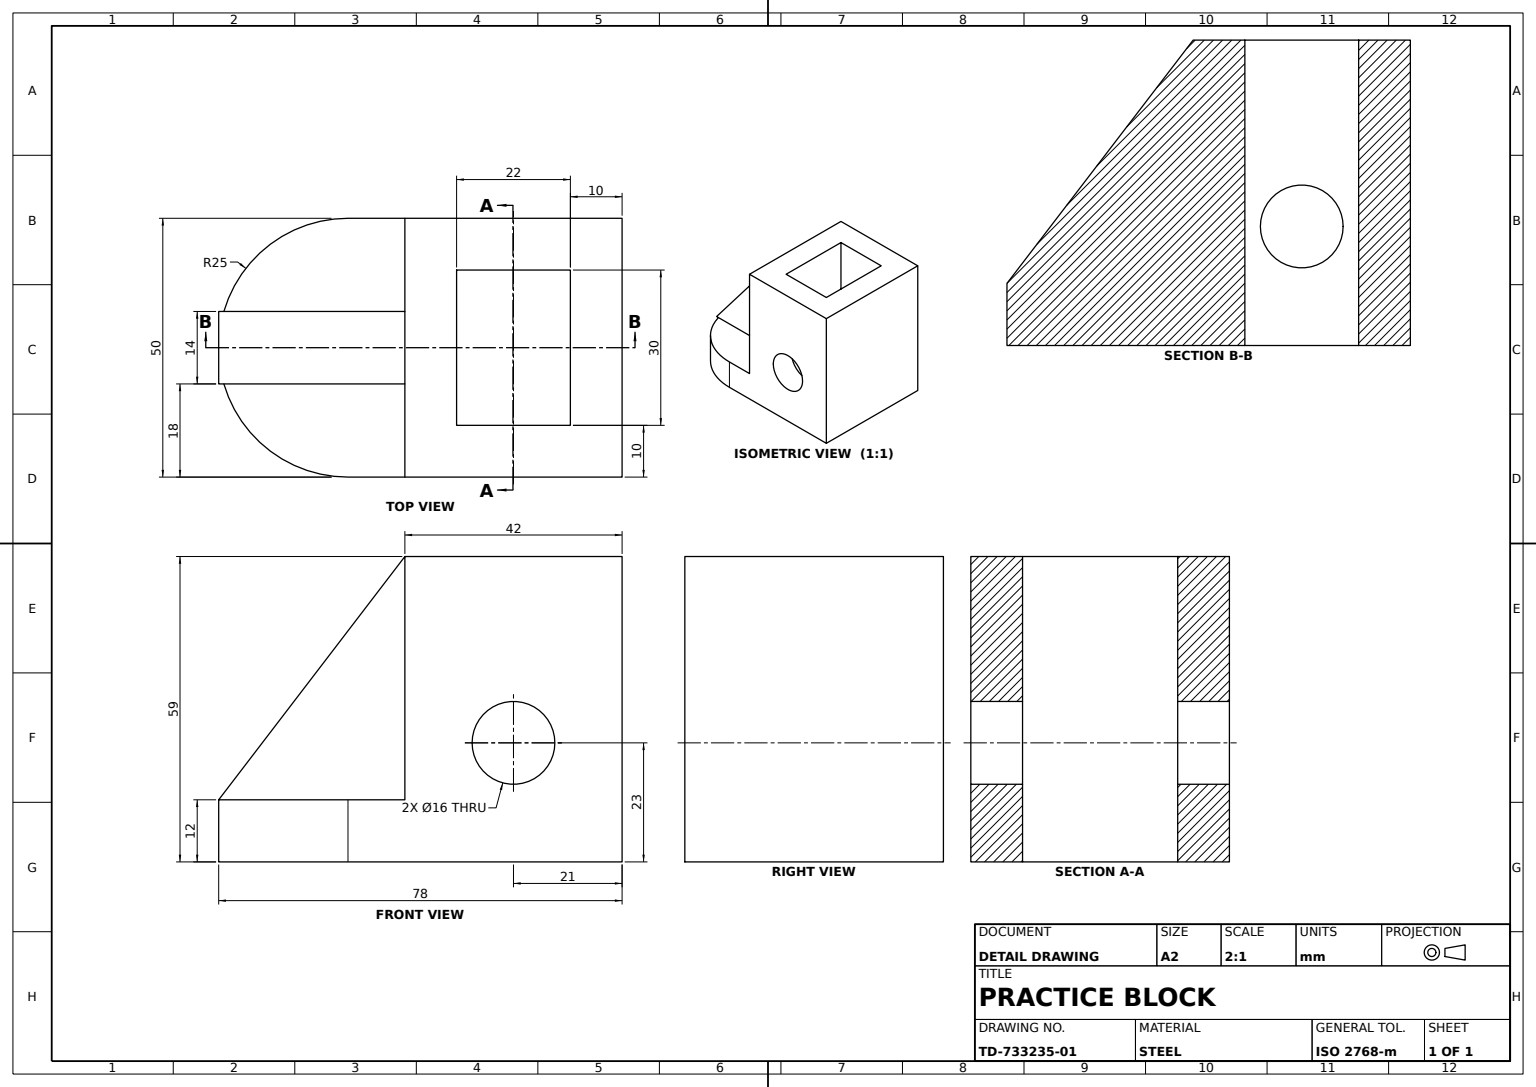
from build123d import *

# Parameters (mm, degrees)
BASE_BLOCK_SKETCH_W              = 78
BASE_BLOCK_SKETCH_H              = 12
BASE_BLOCK_DEPTH                 = 50
UPPER_BLOCK_SKETCH_W             = 50
UPPER_BLOCK_SKETCH_H             = 47
UPPER_BLOCK_DEPTH                = 42
STEP_CUT_12MM_DEPTH              = 12
CROSS_HOLE_SKETCH_R              = 8
CROSS_HOLE_DEPTH                 = 50
RECTANGULAR_POCKET_SKETCH_W      = 22
RECTANGULAR_POCKET_SKETCH_H      = 30
RECTANGULAR_THROUGH_POCKET_DEPTH = 80
WEDGE_LUG_DEPTH                  = 50
WEDGE_CUT_A_DEPTH                = 18
WEDGE_CUT_B_DEPTH                = 18


with BuildPart() as part:
    # Base Block Sketch → Base Block (new body)
    with BuildSketch(Plane.XY):
        with Locations((39, -6)):
            Rectangle(BASE_BLOCK_SKETCH_W, BASE_BLOCK_SKETCH_H)
    extrude(amount=BASE_BLOCK_DEPTH)

    # Upper Block Sketch → Upper Block (add)
    with BuildSketch(Plane(origin=(78, 0, 0), x_dir=(0, 0, -1), z_dir=(1, 0, 0))):
        with Locations((-25, 23.5)):
            Rectangle(UPPER_BLOCK_SKETCH_W, UPPER_BLOCK_SKETCH_H)
    extrude(amount=-UPPER_BLOCK_DEPTH)

    # Step Cut Sketch → Step Cut 12mm (cut)
    with BuildSketch(Plane(origin=(0, 0, 0), x_dir=(1, 0, 0), z_dir=(0, 1, 0))):
        with BuildLine():
            Line((25, 0), (0, 0))
            Line((0, 0), (0, -25))
            ThreePointArc((0, -25), (7.32233047, -7.32233047), (25, 0))
        make_face()
        with BuildLine():
            ThreePointArc((25, -50), (7.32233047, -42.67766953), (0, -25))
            Line((0, -25), (0, -50))
            Line((0, -50), (25, -50))
        make_face()
    extrude(amount=-STEP_CUT_12MM_DEPTH, mode=Mode.SUBTRACT)

    # Cross Hole Sketch → Cross Hole (cut)
    with BuildSketch(Plane.XY.offset(50)):
        with Locations((57, 11)):
            Circle(CROSS_HOLE_SKETCH_R)
    extrude(amount=-CROSS_HOLE_DEPTH, mode=Mode.SUBTRACT)

    # Rectangular Pocket Sketch → Rectangular Through Pocket (cut)
    with BuildSketch(Plane(origin=(0, 47, 0), x_dir=(1, 0, 0), z_dir=(0, 1, 0))):
        with Locations((57, -25)):
            Rectangle(RECTANGULAR_POCKET_SKETCH_W, RECTANGULAR_POCKET_SKETCH_H)
    extrude(amount=-RECTANGULAR_THROUGH_POCKET_DEPTH, mode=Mode.SUBTRACT)

    # Wedge Lug Sketch → Wedge Lug (add)
    with BuildSketch(Plane.XY.offset(50)):
        Polygon((36, 47), (0, 0), (36, 0), align=None)
    extrude(amount=-WEDGE_LUG_DEPTH)

    # Wedge Cut A Sketch → Wedge Cut A (cut)
    with BuildSketch(Plane.XY.offset(50)):
        Polygon((36, 47), (36, 0), (0, 0), align=None)
    extrude(amount=-WEDGE_CUT_A_DEPTH, mode=Mode.SUBTRACT)

    # Wedge Cut B Sketch → Wedge Cut B (cut)
    with BuildSketch(Plane(origin=(0, 0, 0), x_dir=(-1, 0, 0), z_dir=(0, 0, -1))):
        Polygon((-36, 47), (-36, 0), (0, 0), align=None)
    extrude(amount=-WEDGE_CUT_B_DEPTH, mode=Mode.SUBTRACT)


solid = part.part
